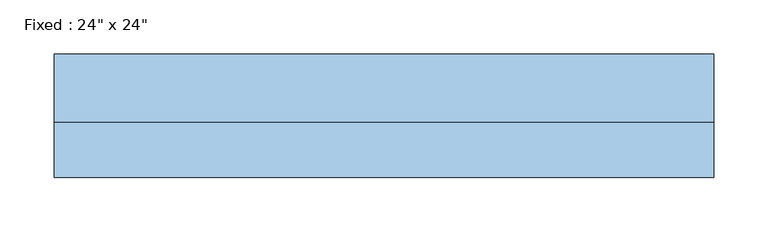
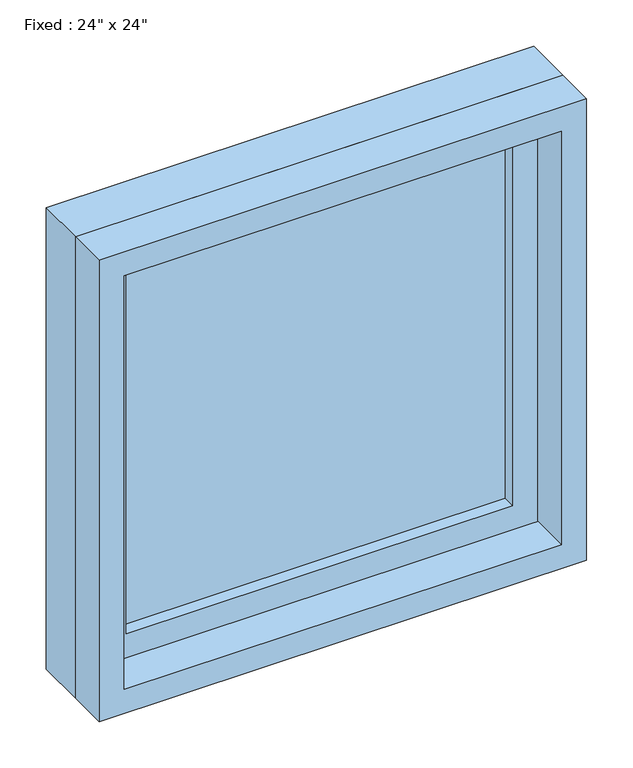
"""IFC4 building model written with IfcOpenShell, lengths in millimetres: window geometry."""

from ifc_helpers import new_model, si_unit, frame, origin, place, context, project, spatial, polyline, outline, extrude, source, transform, mapped, element, save


def window_0e670d86(model_context):
    return source(origin(), model_context, "Body", "SweptSolid", [
        extrude(outline(polyline([(203.2, 9.525), (-279.4, 9.525), (-279.4, 22.225), (203.2, 22.225), (203.2, 9.525)])), frame((0.0, 0.0, 977.9), z_axis=(0.0, 0.0, 1.0), x_axis=(1.0, 0.0, 0.0)), (0.0, 0.0, 1.0), 482.6),
        extrude(outline(polyline([(1504.95, -323.85), (933.45, -323.85), (933.45, 247.65), (1504.95, 247.65), (1504.95, -323.85)]), holes=[polyline([(1460.5, -279.4), (1460.5, 203.2), (977.9, 203.2), (977.9, -279.4), (1460.5, -279.4)])]), frame((0.0, -6.35, 0.0), z_axis=(0.0, 1.0, 0.0), x_axis=(0.0, 0.0, 1.0)), (0.0, 0.0, 1.0), 44.45),
        extrude(outline(polyline([(1524.0, -342.9), (914.4, -342.9), (914.4, 266.7), (1524.0, 266.7), (1524.0, -342.9)]), holes=[polyline([(1492.25, -311.15), (1492.25, 234.95), (946.15, 234.95), (946.15, -311.15), (1492.25, -311.15)])]), frame((0.0, -57.15, 0.0), z_axis=(0.0, 1.0, 0.0), x_axis=(0.0, 0.0, 1.0)), (0.0, 0.0, 1.0), 50.8),
        extrude(outline(polyline([(1524.0, 266.7), (1524.0, -342.9), (914.4, -342.9), (914.4, 266.7), (1524.0, 266.7)]), holes=[polyline([(1504.95, 247.65), (933.45, 247.65), (933.45, -323.85), (1504.95, -323.85), (1504.95, 247.65)])]), frame((0.0, -6.35, 0.0), z_axis=(0.0, 1.0, 0.0), x_axis=(0.0, 0.0, 1.0)), (0.0, 0.0, 1.0), 63.5),
    ])


if __name__ == "__main__":
    model = new_model("IFC4")
    model_context = context("Model", 3, world=origin())
    ifc_project = project(units=[si_unit("LENGTHUNIT", "METRE", prefix="MILLI")], contexts=[model_context])
    site = spatial("IfcSite", under=ifc_project)
    building = spatial("IfcBuilding", under=site)
    placement = place(None, origin())
    window_shape = window_0e670d86(model_context)
    element("IfcWindow", 1, ObjectType="Fixed : 24\" x 24\"", at=placement, inside=building, context=model_context, shape_type="MappedRepresentation", body=[
        mapped(window_shape, transform((0.0, 0.0, 0.0), x_axis=(1.0, 0.0, 0.0), y_axis=(0.0, 1.0, 0.0), z_axis=(0.0, 0.0, 1.0))),
    ])
    save(model, "model.ifc")

# Revit data of these elements
# Type "Fixed : 24\" x 24\""
#   Type Mark = "3"
#   Construction Type Id = "GSP4R"
#   Assembly Code = "B2020100"
#   Analytic Construction = "1/8 in Pilkington single glazing"
#   Visual Light Transmittance = 0.9
#   Solar Heat Gain Coefficient = 0.78
#   Heat Transfer Coefficient (U) = 0.6496 BTU/(h·ft²·°F)
#   Height = 2' - 0"
#   Default Sill Height = 3' - 0"
#   Width = 2' - 0"
#   Window Inset = 0' - 0 3/4"
#   Define Thermal Properties by = 1
#   Define Thermal Properties by = 1
#   Glass Pane Material = Glass
#   Sash Material = Sash
#   Wall Closure = (empty or 0)
# Element 1 (IfcWindow, "Fixed : 24\" x 24\"")
#   Materials on its faces: "Sash", "Glass"
# Materials
#   "Glass": class "Glass", colour RGB 0 128 192, transparency 0.75, Description = "Soda Lime Glass", Cost = 0
#   "Sash": class "Wood", colour RGB 224 178 126, transparency 0, Cost = 0
